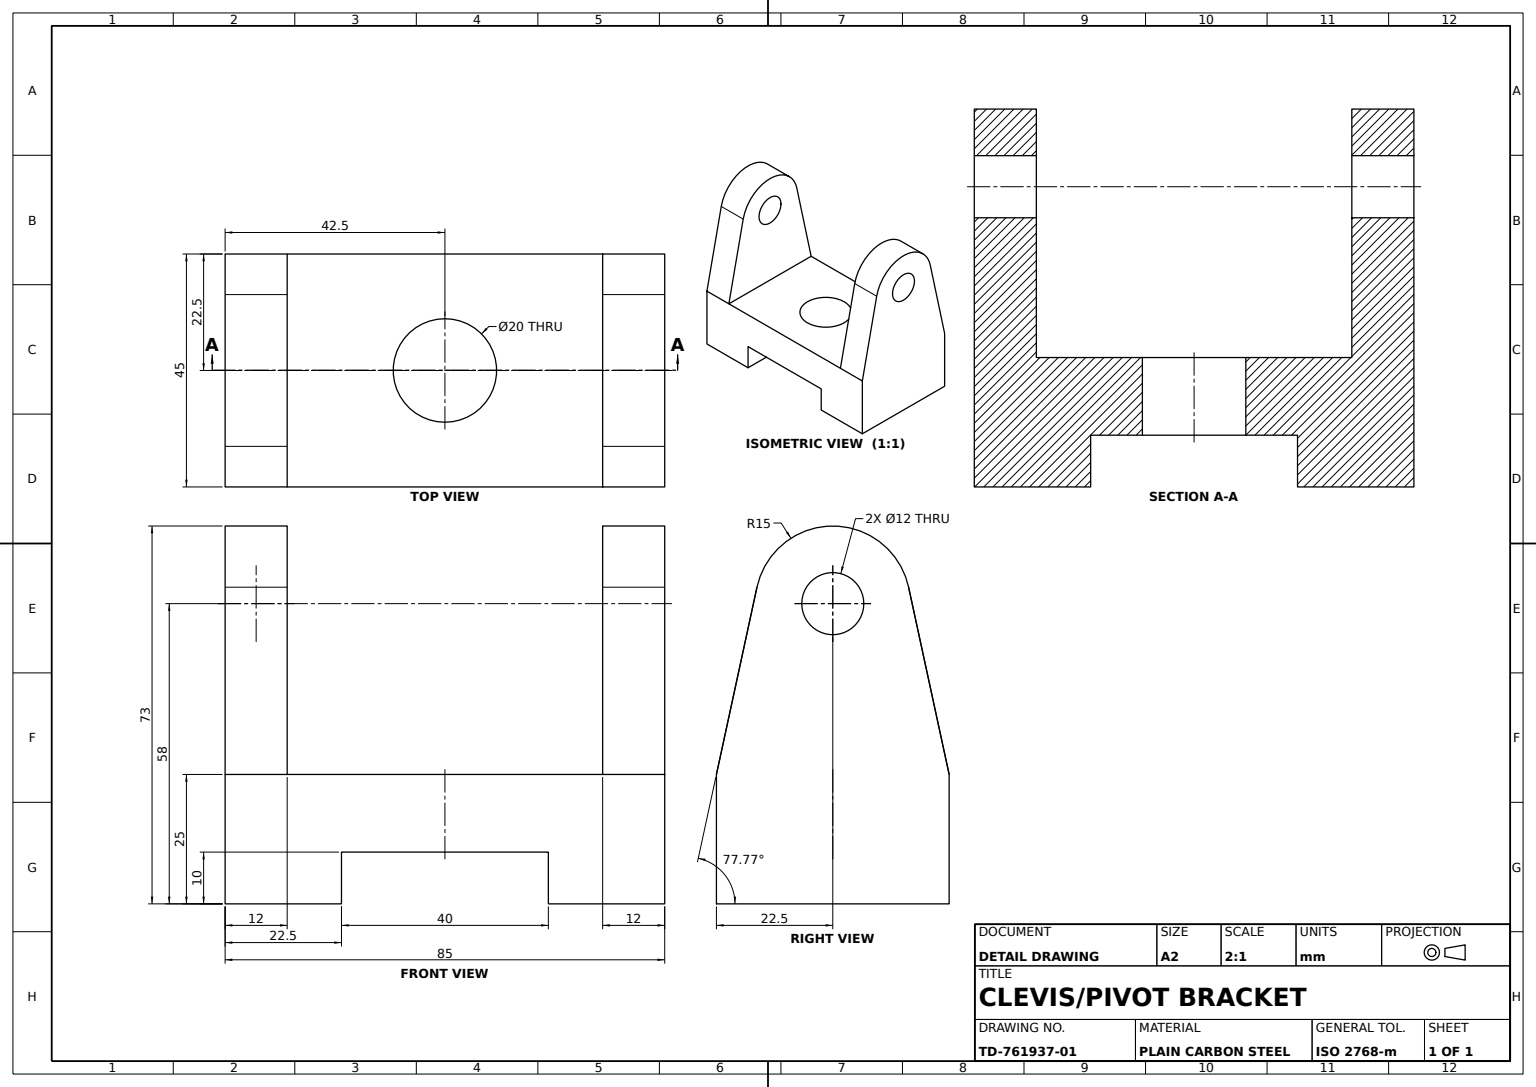
from build123d import *

# Parameters (mm, degrees)
T_SLOT_BASE_DEPTH      = 45
CENTRE_BORE_SKETCH_R   = 10
CENTRE_BORE_20_DEPTH   = 45
CLEVIS_LUG_1_PROFILE_R = 6
CLEVIS_LUG_1_DEPTH     = 12
CLEVIS_START           = -12
CLEVIS_LUG_2_PROFILE_R = 6
CLEVIS_LUG_2_DEPTH     = 12


with BuildPart() as part:
    # T-Slot Base Profile → T-Slot Base (new body)
    with BuildSketch(Plane.XY):
        Polygon((-20, 0), (-42.5, 0), (-42.5, 25), (42.5, 25), (42.5, 0), (20, 0), (20, 10), (-20, 10), align=None)
    extrude(amount=T_SLOT_BASE_DEPTH)

    # Centre Bore Sketch → Centre Bore Ø20 (cut)
    with BuildSketch(Plane(origin=(0, 25, 0), x_dir=(1, 0, 0), z_dir=(0, 1, 0))):
        with Locations(Location((0, -22.5, 0), (0, 0, 270))):
            Circle(CENTRE_BORE_SKETCH_R)
    extrude(amount=-CENTRE_BORE_20_DEPTH, mode=Mode.SUBTRACT)

    # Clevis Lug 1 Profile → Clevis Lug 1 (add)
    with BuildSketch(Plane.ZY.offset(42.5)):
        with BuildLine():
            Line((0, 25), (45, 25))
            Line((45, 25), (37.159683171, 61.177056708))
            ThreePointArc((37.159683171, 61.177056708), (22.5, 73), (7.840316829, 61.177056708))
            Line((7.840316829, 61.177056708), (0, 25))
        make_face()
        with Locations((22.5, 58)):
            Circle(CLEVIS_LUG_1_PROFILE_R, mode=Mode.SUBTRACT)
    extrude(amount=-CLEVIS_LUG_1_DEPTH)

    # Clevis Lug 2 Profile → Clevis Lug 2 (add)
    with BuildSketch(Plane(origin=(42.5, 0, 0), x_dir=(0, 0, -1), z_dir=(1, 0, 0)).offset(CLEVIS_START)):
        with BuildLine():
            Line((-37.159683171, 61.177056708), (-45, 25))
            Line((-45, 25), (0, 25))
            Line((0, 25), (-7.840316829, 61.177056708))
            ThreePointArc((-7.840316829, 61.177056708), (-22.5, 73), (-37.159683171, 61.177056708))
        make_face()
        with Locations(Location((-22.5, 58, 0), (0, 0, 180))):
            Circle(CLEVIS_LUG_2_PROFILE_R, mode=Mode.SUBTRACT)
    extrude(amount=CLEVIS_LUG_2_DEPTH)


solid = part.part
